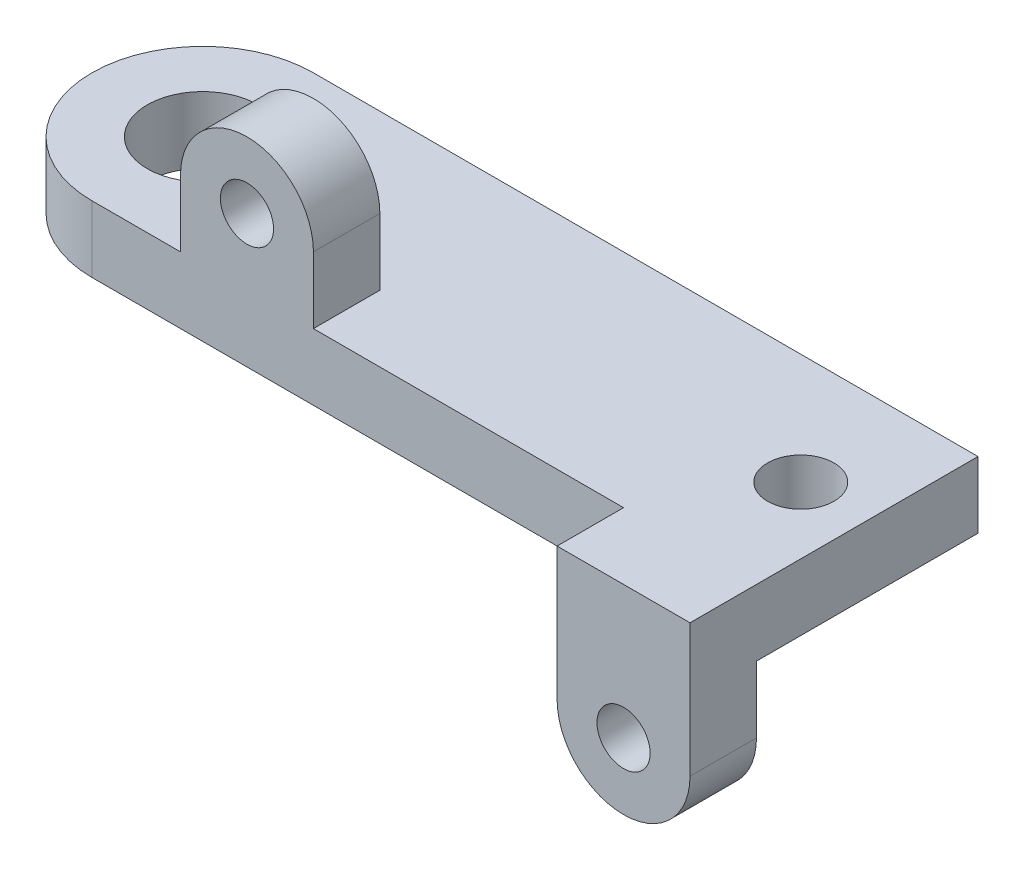
ISO-10303-21;
HEADER;
FILE_DESCRIPTION(('STEP AP214'),'2;1');
FILE_NAME('part.step','',(''),(''),'','','');
FILE_SCHEMA(('AUTOMOTIVE_DESIGN { 1 0 10303 214 1 1 1 1 }'));
ENDSEC;
DATA;
#1=APPLICATION_CONTEXT('core data for automotive mechanical design processes');
#2=APPLICATION_PROTOCOL_DEFINITION('international standard','automotive_design',2000,#1);
#3=PRODUCT_CONTEXT('',#1,'mechanical');
#4=PRODUCT('Part','Part','',(#3));
#5=PRODUCT_RELATED_PRODUCT_CATEGORY('part','',(#4));
#6=PRODUCT_DEFINITION_FORMATION('','',#4);
#7=PRODUCT_DEFINITION_CONTEXT('part definition',#1,'design');
#8=PRODUCT_DEFINITION('design','',#6,#7);
#9=PRODUCT_DEFINITION_SHAPE('','',#8);
#10=(LENGTH_UNIT() NAMED_UNIT(*) SI_UNIT(.MILLI.,.METRE.));
#11=(NAMED_UNIT(*) PLANE_ANGLE_UNIT() SI_UNIT($,.RADIAN.));
#12=(NAMED_UNIT(*) SI_UNIT($,.STERADIAN.) SOLID_ANGLE_UNIT());
#13=UNCERTAINTY_MEASURE_WITH_UNIT(LENGTH_MEASURE(1.E-05),#10,'distance_accuracy_value','');
#14=(GEOMETRIC_REPRESENTATION_CONTEXT(3) GLOBAL_UNCERTAINTY_ASSIGNED_CONTEXT((#13)) GLOBAL_UNIT_ASSIGNED_CONTEXT((#10,
#11,#12)) REPRESENTATION_CONTEXT('',''));
#15=CARTESIAN_POINT('',(0.,0.,0.));
#16=DIRECTION('',(0.,0.,1.));
#17=DIRECTION('',(1.,0.,0.));
#18=AXIS2_PLACEMENT_3D('',#15,#16,#17);
#19=CARTESIAN_POINT('',(120.,-45.,0.));
#20=DIRECTION('',(1.,0.,0.));
#21=DIRECTION('',(0.,0.,-1.));
#22=AXIS2_PLACEMENT_3D('',#19,#20,#21);
#23=PLANE('',#22);
#24=DIRECTION('',(0.,0.,1.));
#25=VECTOR('',#24,1.);
#26=CARTESIAN_POINT('',(120.,-30.,-4.99999999999994));
#27=LINE('',#26,#25);
#28=CARTESIAN_POINT('',(120.,-30.,25.));
#29=VERTEX_POINT('',#28);
#30=CARTESIAN_POINT('',(120.,-30.,40.));
#31=VERTEX_POINT('',#30);
#32=EDGE_CURVE('E165',#29,#31,#27,.T.);
#33=ORIENTED_EDGE('',*,*,#32,.T.);
#34=DIRECTION('',(0.,1.,0.));
#35=VECTOR('',#34,1.);
#36=CARTESIAN_POINT('',(120.,-45.,40.));
#37=LINE('',#36,#35);
#38=CARTESIAN_POINT('',(120.,0.,40.));
#39=VERTEX_POINT('',#38);
#40=EDGE_CURVE('E186',#31,#39,#37,.T.);
#41=ORIENTED_EDGE('',*,*,#40,.T.);
#42=DIRECTION('',(0.,0.,-1.));
#43=VECTOR('',#42,1.);
#44=CARTESIAN_POINT('',(120.,0.,0.));
#45=LINE('',#44,#43);
#46=CARTESIAN_POINT('',(120.,0.,25.));
#47=VERTEX_POINT('',#46);
#48=EDGE_CURVE('E177',#39,#47,#45,.T.);
#49=ORIENTED_EDGE('',*,*,#48,.T.);
#50=DIRECTION('',(0.,1.,0.));
#51=VECTOR('',#50,1.);
#52=CARTESIAN_POINT('',(120.,-45.,25.));
#53=LINE('',#52,#51);
#54=CARTESIAN_POINT('',(120.,-15.,25.));
#55=VERTEX_POINT('',#54);
#56=EDGE_CURVE('E185',#55,#47,#53,.T.);
#57=ORIENTED_EDGE('',*,*,#56,.F.);
#58=EDGE_CURVE('E189',#29,#55,#53,.T.);
#59=ORIENTED_EDGE('',*,*,#58,.F.);
#60=EDGE_LOOP('',(#33,#41,#49,#57,#59));
#61=FACE_BOUND('',#60,.T.);
#62=ADVANCED_FACE('F41',(#61),#23,.F.);
#63=CARTESIAN_POINT('',(0.,-15.,25.));
#64=DIRECTION('',(0.,0.,-1.));
#65=DIRECTION('',(-1.,0.,0.));
#66=AXIS2_PLACEMENT_3D('',#63,#64,#65);
#67=PLANE('',#66);
#68=DIRECTION('',(-1.,0.,0.));
#69=VECTOR('',#68,1.);
#70=CARTESIAN_POINT('',(0.,0.,25.));
#71=LINE('',#70,#69);
#72=CARTESIAN_POINT('',(50.,0.,25.));
#73=VERTEX_POINT('',#72);
#74=EDGE_CURVE('E223',#47,#73,#71,.T.);
#75=ORIENTED_EDGE('',*,*,#74,.T.);
#76=DIRECTION('',(0.,1.,0.));
#77=VECTOR('',#76,1.);
#78=CARTESIAN_POINT('',(50.,-3.36192289386007,25.));
#79=LINE('',#78,#77);
#80=CARTESIAN_POINT('',(50.,15.,25.));
#81=VERTEX_POINT('',#80);
#82=EDGE_CURVE('E147',#73,#81,#79,.T.);
#83=ORIENTED_EDGE('',*,*,#82,.T.);
#84=CARTESIAN_POINT('',(35.,15.,25.));
#85=DIRECTION('',(0.,0.,1.));
#86=DIRECTION('',(1.,0.,0.));
#87=AXIS2_PLACEMENT_3D('',#84,#85,#86);
#88=CIRCLE('',#87,15.);
#89=CARTESIAN_POINT('',(20.,15.,25.));
#90=VERTEX_POINT('',#89);
#91=EDGE_CURVE('E158',#81,#90,#88,.T.);
#92=ORIENTED_EDGE('',*,*,#91,.T.);
#93=DIRECTION('',(0.,-1.,0.));
#94=VECTOR('',#93,1.);
#95=CARTESIAN_POINT('',(20.,15.,25.));
#96=LINE('',#95,#94);
#97=CARTESIAN_POINT('',(20.,0.,25.));
#98=VERTEX_POINT('',#97);
#99=EDGE_CURVE('E57',#90,#98,#96,.T.);
#100=ORIENTED_EDGE('',*,*,#99,.T.);
#101=CARTESIAN_POINT('',(0.,0.,25.));
#102=VERTEX_POINT('',#101);
#103=EDGE_CURVE('E221',#98,#102,#71,.T.);
#104=ORIENTED_EDGE('',*,*,#103,.T.);
#105=DIRECTION('',(0.,1.,0.));
#106=VECTOR('',#105,1.);
#107=CARTESIAN_POINT('',(0.,-15.,25.));
#108=LINE('',#107,#106);
#109=CARTESIAN_POINT('',(0.,-15.,25.));
#110=VERTEX_POINT('',#109);
#111=EDGE_CURVE('E233',#110,#102,#108,.T.);
#112=ORIENTED_EDGE('',*,*,#111,.F.);
#113=DIRECTION('',(-1.,0.,0.));
#114=VECTOR('',#113,1.);
#115=CARTESIAN_POINT('',(0.,-15.,25.));
#116=LINE('',#115,#114);
#117=EDGE_CURVE('E202',#55,#110,#116,.T.);
#118=ORIENTED_EDGE('',*,*,#117,.F.);
#119=ORIENTED_EDGE('',*,*,#56,.T.);
#120=EDGE_LOOP('',(#75,#83,#92,#100,#104,#112,#118,#119));
#121=FACE_BOUND('',#120,.T.);
#122=CARTESIAN_POINT('',(35.,15.,25.));
#123=DIRECTION('',(0.,0.,1.));
#124=DIRECTION('',(1.,0.,0.));
#125=AXIS2_PLACEMENT_3D('',#122,#123,#124);
#126=CIRCLE('',#125,6.);
#127=CARTESIAN_POINT('',(41.,15.,25.));
#128=VERTEX_POINT('',#127);
#129=EDGE_CURVE('E152',#128,#128,#126,.T.);
#130=ORIENTED_EDGE('',*,*,#129,.F.);
#131=EDGE_LOOP('',(#130));
#132=FACE_BOUND('',#131,.T.);
#133=ADVANCED_FACE('F244',(#121,#132),#67,.F.);
#134=CARTESIAN_POINT('',(0.,-15.,-25.));
#135=DIRECTION('',(0.,0.,1.));
#136=DIRECTION('',(1.,0.,0.));
#137=AXIS2_PLACEMENT_3D('',#134,#135,#136);
#138=PLANE('',#137);
#139=DIRECTION('',(1.,0.,0.));
#140=VECTOR('',#139,1.);
#141=CARTESIAN_POINT('',(0.,0.,-25.));
#142=LINE('',#141,#140);
#143=CARTESIAN_POINT('',(0.,0.,-25.));
#144=VERTEX_POINT('',#143);
#145=CARTESIAN_POINT('',(150.,0.,-25.));
#146=VERTEX_POINT('',#145);
#147=EDGE_CURVE('E217',#144,#146,#142,.T.);
#148=ORIENTED_EDGE('',*,*,#147,.T.);
#149=DIRECTION('',(0.,1.,0.));
#150=VECTOR('',#149,1.);
#151=CARTESIAN_POINT('',(150.,-15.,-25.));
#152=LINE('',#151,#150);
#153=CARTESIAN_POINT('',(150.,-15.,-25.));
#154=VERTEX_POINT('',#153);
#155=EDGE_CURVE('E229',#154,#146,#152,.T.);
#156=ORIENTED_EDGE('',*,*,#155,.F.);
#157=DIRECTION('',(1.,0.,0.));
#158=VECTOR('',#157,1.);
#159=CARTESIAN_POINT('',(0.,-15.,-25.));
#160=LINE('',#159,#158);
#161=CARTESIAN_POINT('',(0.,-15.,-25.));
#162=VERTEX_POINT('',#161);
#163=EDGE_CURVE('E200',#162,#154,#160,.T.);
#164=ORIENTED_EDGE('',*,*,#163,.F.);
#165=DIRECTION('',(0.,1.,0.));
#166=VECTOR('',#165,1.);
#167=CARTESIAN_POINT('',(0.,-15.,-25.));
#168=LINE('',#167,#166);
#169=EDGE_CURVE('E215',#162,#144,#168,.T.);
#170=ORIENTED_EDGE('',*,*,#169,.T.);
#171=EDGE_LOOP('',(#148,#156,#164,#170));
#172=FACE_BOUND('',#171,.T.);
#173=ADVANCED_FACE('F285',(#172),#138,.F.);
#174=CARTESIAN_POINT('',(150.,-15.,0.));
#175=DIRECTION('',(-1.,0.,0.));
#176=DIRECTION('',(0.,0.,1.));
#177=AXIS2_PLACEMENT_3D('',#174,#175,#176);
#178=PLANE('',#177);
#179=DIRECTION('',(0.,1.,0.));
#180=VECTOR('',#179,1.);
#181=CARTESIAN_POINT('',(150.,-45.,40.));
#182=LINE('',#181,#180);
#183=CARTESIAN_POINT('',(150.,-30.,40.0000000000001));
#184=VERTEX_POINT('',#183);
#185=CARTESIAN_POINT('',(150.,0.,40.));
#186=VERTEX_POINT('',#185);
#187=EDGE_CURVE('E188',#184,#186,#182,.T.);
#188=ORIENTED_EDGE('',*,*,#187,.F.);
#189=DIRECTION('',(0.,0.,1.));
#190=VECTOR('',#189,1.);
#191=CARTESIAN_POINT('',(150.,-30.,-4.99999999999994));
#192=LINE('',#191,#190);
#193=CARTESIAN_POINT('',(150.,-30.,25.));
#194=VERTEX_POINT('',#193);
#195=EDGE_CURVE('E163',#194,#184,#192,.T.);
#196=ORIENTED_EDGE('',*,*,#195,.F.);
#197=DIRECTION('',(0.,1.,0.));
#198=VECTOR('',#197,1.);
#199=CARTESIAN_POINT('',(150.,-45.,25.));
#200=LINE('',#199,#198);
#201=CARTESIAN_POINT('',(150.,-15.,25.));
#202=VERTEX_POINT('',#201);
#203=EDGE_CURVE('E181',#194,#202,#200,.T.);
#204=ORIENTED_EDGE('',*,*,#203,.T.);
#205=DIRECTION('',(0.,0.,1.));
#206=VECTOR('',#205,1.);
#207=CARTESIAN_POINT('',(150.,-15.,0.));
#208=LINE('',#207,#206);
#209=EDGE_CURVE('E207',#154,#202,#208,.T.);
#210=ORIENTED_EDGE('',*,*,#209,.F.);
#211=ORIENTED_EDGE('',*,*,#155,.T.);
#212=DIRECTION('',(0.,0.,1.));
#213=VECTOR('',#212,1.);
#214=CARTESIAN_POINT('',(150.,0.,0.));
#215=LINE('',#214,#213);
#216=EDGE_CURVE('E198',#146,#186,#215,.T.);
#217=ORIENTED_EDGE('',*,*,#216,.T.);
#218=EDGE_LOOP('',(#188,#196,#204,#210,#211,#217));
#219=FACE_BOUND('',#218,.T.);
#220=ADVANCED_FACE('F298',(#219),#178,.F.);
#221=CARTESIAN_POINT('',(0.,-15.,0.));
#222=DIRECTION('',(0.,1.,0.));
#223=DIRECTION('',(0.,0.,1.));
#224=AXIS2_PLACEMENT_3D('',#221,#222,#223);
#225=CYLINDRICAL_SURFACE('',#224,12.5);
#226=CARTESIAN_POINT('',(0.,-15.,0.));
#227=DIRECTION('',(0.,1.,0.));
#228=DIRECTION('',(0.,0.,1.));
#229=AXIS2_PLACEMENT_3D('',#226,#227,#228);
#230=CIRCLE('',#229,12.5);
#231=CARTESIAN_POINT('',(0.,-15.,12.5));
#232=VERTEX_POINT('',#231);
#233=EDGE_CURVE('E191',#232,#232,#230,.T.);
#234=ORIENTED_EDGE('',*,*,#233,.F.);
#235=EDGE_LOOP('',(#234));
#236=FACE_BOUND('',#235,.T.);
#237=CARTESIAN_POINT('',(0.,0.,0.));
#238=DIRECTION('',(0.,1.,0.));
#239=DIRECTION('',(0.,0.,1.));
#240=AXIS2_PLACEMENT_3D('',#237,#238,#239);
#241=CIRCLE('',#240,12.5);
#242=CARTESIAN_POINT('',(0.,0.,12.5));
#243=VERTEX_POINT('',#242);
#244=EDGE_CURVE('E214',#243,#243,#241,.T.);
#245=ORIENTED_EDGE('',*,*,#244,.T.);
#246=EDGE_LOOP('',(#245));
#247=FACE_BOUND('',#246,.T.);
#248=ADVANCED_FACE('F300',(#236,#247),#225,.F.);
#249=CARTESIAN_POINT('',(135.,-15.,0.));
#250=DIRECTION('',(0.,1.,0.));
#251=DIRECTION('',(0.,0.,1.));
#252=AXIS2_PLACEMENT_3D('',#249,#250,#251);
#253=CYLINDRICAL_SURFACE('',#252,7.50000000000001);
#254=CARTESIAN_POINT('',(135.,-15.,0.));
#255=DIRECTION('',(0.,1.,0.));
#256=DIRECTION('',(0.,0.,1.));
#257=AXIS2_PLACEMENT_3D('',#254,#255,#256);
#258=CIRCLE('',#257,7.50000000000001);
#259=CARTESIAN_POINT('',(135.,-15.,7.50000000000002));
#260=VERTEX_POINT('',#259);
#261=EDGE_CURVE('E195',#260,#260,#258,.T.);
#262=ORIENTED_EDGE('',*,*,#261,.F.);
#263=EDGE_LOOP('',(#262));
#264=FACE_BOUND('',#263,.T.);
#265=CARTESIAN_POINT('',(135.,0.,0.));
#266=DIRECTION('',(0.,1.,0.));
#267=DIRECTION('',(0.,0.,1.));
#268=AXIS2_PLACEMENT_3D('',#265,#266,#267);
#269=CIRCLE('',#268,7.50000000000001);
#270=CARTESIAN_POINT('',(135.,0.,7.50000000000002));
#271=VERTEX_POINT('',#270);
#272=EDGE_CURVE('E183',#271,#271,#269,.T.);
#273=ORIENTED_EDGE('',*,*,#272,.T.);
#274=EDGE_LOOP('',(#273));
#275=FACE_BOUND('',#274,.T.);
#276=ADVANCED_FACE('F43',(#264,#275),#253,.F.);
#277=CARTESIAN_POINT('',(0.,-15.,0.));
#278=DIRECTION('',(0.,1.,0.));
#279=DIRECTION('',(0.,0.,1.));
#280=AXIS2_PLACEMENT_3D('',#277,#278,#279);
#281=CYLINDRICAL_SURFACE('',#280,25.);
#282=CARTESIAN_POINT('',(0.,0.,0.));
#283=DIRECTION('',(0.,1.,0.));
#284=DIRECTION('',(0.,0.,1.));
#285=AXIS2_PLACEMENT_3D('',#282,#283,#284);
#286=CIRCLE('',#285,25.);
#287=EDGE_CURVE('E222',#144,#102,#286,.T.);
#288=ORIENTED_EDGE('',*,*,#287,.F.);
#289=ORIENTED_EDGE('',*,*,#169,.F.);
#290=CARTESIAN_POINT('',(0.,-15.,0.));
#291=DIRECTION('',(0.,1.,0.));
#292=DIRECTION('',(0.,0.,1.));
#293=AXIS2_PLACEMENT_3D('',#290,#291,#292);
#294=CIRCLE('',#293,25.);
#295=EDGE_CURVE('E205',#162,#110,#294,.T.);
#296=ORIENTED_EDGE('',*,*,#295,.T.);
#297=ORIENTED_EDGE('',*,*,#111,.T.);
#298=EDGE_LOOP('',(#288,#289,#296,#297));
#299=FACE_BOUND('',#298,.T.);
#300=ADVANCED_FACE('F249',(#299),#281,.T.);
#301=CARTESIAN_POINT('',(0.,-15.,0.));
#302=DIRECTION('',(0.,1.,0.));
#303=DIRECTION('',(0.,0.,1.));
#304=AXIS2_PLACEMENT_3D('',#301,#302,#303);
#305=PLANE('',#304);
#306=ORIENTED_EDGE('',*,*,#261,.T.);
#307=EDGE_LOOP('',(#306));
#308=FACE_BOUND('',#307,.T.);
#309=ORIENTED_EDGE('',*,*,#233,.T.);
#310=EDGE_LOOP('',(#309));
#311=FACE_BOUND('',#310,.T.);
#312=ORIENTED_EDGE('',*,*,#163,.T.);
#313=ORIENTED_EDGE('',*,*,#209,.T.);
#314=EDGE_CURVE('E206',#202,#55,#116,.T.);
#315=ORIENTED_EDGE('',*,*,#314,.T.);
#316=ORIENTED_EDGE('',*,*,#117,.T.);
#317=ORIENTED_EDGE('',*,*,#295,.F.);
#318=EDGE_LOOP('',(#312,#313,#315,#316,#317));
#319=FACE_BOUND('',#318,.T.);
#320=ADVANCED_FACE('F251',(#308,#311,#319),#305,.F.);
#321=CARTESIAN_POINT('',(0.,0.,0.));
#322=DIRECTION('',(0.,1.,0.));
#323=DIRECTION('',(0.,0.,1.));
#324=AXIS2_PLACEMENT_3D('',#321,#322,#323);
#325=PLANE('',#324);
#326=DIRECTION('',(0.,0.,-1.));
#327=VECTOR('',#326,1.);
#328=CARTESIAN_POINT('',(50.,0.,0.));
#329=LINE('',#328,#327);
#330=CARTESIAN_POINT('',(50.,0.,10.));
#331=VERTEX_POINT('',#330);
#332=EDGE_CURVE('E11',#73,#331,#329,.T.);
#333=ORIENTED_EDGE('',*,*,#332,.F.);
#334=ORIENTED_EDGE('',*,*,#74,.F.);
#335=ORIENTED_EDGE('',*,*,#48,.F.);
#336=DIRECTION('',(-1.,0.,0.));
#337=VECTOR('',#336,1.);
#338=CARTESIAN_POINT('',(0.,0.,40.0000000000001));
#339=LINE('',#338,#337);
#340=EDGE_CURVE('E179',#186,#39,#339,.T.);
#341=ORIENTED_EDGE('',*,*,#340,.F.);
#342=ORIENTED_EDGE('',*,*,#216,.F.);
#343=ORIENTED_EDGE('',*,*,#147,.F.);
#344=ORIENTED_EDGE('',*,*,#287,.T.);
#345=ORIENTED_EDGE('',*,*,#103,.F.);
#346=DIRECTION('',(0.,0.,1.));
#347=VECTOR('',#346,1.);
#348=CARTESIAN_POINT('',(20.,0.,0.));
#349=LINE('',#348,#347);
#350=CARTESIAN_POINT('',(20.,0.,10.));
#351=VERTEX_POINT('',#350);
#352=EDGE_CURVE('E47',#351,#98,#349,.T.);
#353=ORIENTED_EDGE('',*,*,#352,.F.);
#354=DIRECTION('',(1.,0.,0.));
#355=VECTOR('',#354,1.);
#356=CARTESIAN_POINT('',(0.,0.,10.));
#357=LINE('',#356,#355);
#358=EDGE_CURVE('E144',#351,#331,#357,.T.);
#359=ORIENTED_EDGE('',*,*,#358,.T.);
#360=EDGE_LOOP('',(#333,#334,#335,#341,#342,#343,#344,#345,#353,#359));
#361=FACE_BOUND('',#360,.T.);
#362=ORIENTED_EDGE('',*,*,#272,.F.);
#363=EDGE_LOOP('',(#362));
#364=FACE_BOUND('',#363,.T.);
#365=ORIENTED_EDGE('',*,*,#244,.F.);
#366=EDGE_LOOP('',(#365));
#367=FACE_BOUND('',#366,.T.);
#368=ADVANCED_FACE('F238',(#361,#364,#367),#325,.T.);
#369=CARTESIAN_POINT('',(0.,-45.,25.));
#370=DIRECTION('',(0.,0.,1.));
#371=DIRECTION('',(1.,0.,0.));
#372=AXIS2_PLACEMENT_3D('',#369,#370,#371);
#373=PLANE('',#372);
#374=CARTESIAN_POINT('',(135.,-30.,25.));
#375=DIRECTION('',(0.,0.,1.));
#376=DIRECTION('',(1.,0.,0.));
#377=AXIS2_PLACEMENT_3D('',#374,#375,#376);
#378=CIRCLE('',#377,6.00000000000002);
#379=CARTESIAN_POINT('',(141.,-30.,25.));
#380=VERTEX_POINT('',#379);
#381=EDGE_CURVE('E171',#380,#380,#378,.T.);
#382=ORIENTED_EDGE('',*,*,#381,.T.);
#383=EDGE_LOOP('',(#382));
#384=FACE_BOUND('',#383,.T.);
#385=ORIENTED_EDGE('',*,*,#203,.F.);
#386=CARTESIAN_POINT('',(135.,-30.,25.));
#387=DIRECTION('',(0.,0.,1.));
#388=DIRECTION('',(1.,0.,0.));
#389=AXIS2_PLACEMENT_3D('',#386,#387,#388);
#390=CIRCLE('',#389,15.);
#391=EDGE_CURVE('E173',#194,#29,#390,.F.);
#392=ORIENTED_EDGE('',*,*,#391,.T.);
#393=ORIENTED_EDGE('',*,*,#58,.T.);
#394=ORIENTED_EDGE('',*,*,#314,.F.);
#395=EDGE_LOOP('',(#385,#392,#393,#394));
#396=FACE_BOUND('',#395,.T.);
#397=ADVANCED_FACE('F288',(#384,#396),#373,.F.);
#398=CARTESIAN_POINT('',(0.,-45.,40.0000000000001));
#399=DIRECTION('',(0.,0.,-1.));
#400=DIRECTION('',(-1.,0.,0.));
#401=AXIS2_PLACEMENT_3D('',#398,#399,#400);
#402=PLANE('',#401);
#403=CARTESIAN_POINT('',(135.,-30.,40.0000000000001));
#404=DIRECTION('',(0.,0.,1.));
#405=DIRECTION('',(1.,0.,0.));
#406=AXIS2_PLACEMENT_3D('',#403,#404,#405);
#407=CIRCLE('',#406,6.00000000000002);
#408=CARTESIAN_POINT('',(141.,-30.,40.0000000000001));
#409=VERTEX_POINT('',#408);
#410=EDGE_CURVE('E169',#409,#409,#407,.T.);
#411=ORIENTED_EDGE('',*,*,#410,.F.);
#412=EDGE_LOOP('',(#411));
#413=FACE_BOUND('',#412,.T.);
#414=ORIENTED_EDGE('',*,*,#40,.F.);
#415=CARTESIAN_POINT('',(135.,-30.,40.0000000000001));
#416=DIRECTION('',(0.,0.,-1.));
#417=DIRECTION('',(1.,0.,0.));
#418=AXIS2_PLACEMENT_3D('',#415,#416,#417);
#419=CIRCLE('',#418,15.);
#420=EDGE_CURVE('E62',#184,#31,#419,.T.);
#421=ORIENTED_EDGE('',*,*,#420,.F.);
#422=ORIENTED_EDGE('',*,*,#187,.T.);
#423=ORIENTED_EDGE('',*,*,#340,.T.);
#424=EDGE_LOOP('',(#414,#421,#422,#423));
#425=FACE_BOUND('',#424,.T.);
#426=ADVANCED_FACE('F287',(#413,#425),#402,.F.);
#427=CARTESIAN_POINT('',(135.,-30.,-4.99999999999994));
#428=DIRECTION('',(0.,0.,1.));
#429=DIRECTION('',(1.,0.,0.));
#430=AXIS2_PLACEMENT_3D('',#427,#428,#429);
#431=CYLINDRICAL_SURFACE('',#430,15.);
#432=ORIENTED_EDGE('',*,*,#195,.T.);
#433=ORIENTED_EDGE('',*,*,#420,.T.);
#434=ORIENTED_EDGE('',*,*,#32,.F.);
#435=ORIENTED_EDGE('',*,*,#391,.F.);
#436=EDGE_LOOP('',(#432,#433,#434,#435));
#437=FACE_BOUND('',#436,.T.);
#438=ADVANCED_FACE('F380',(#437),#431,.T.);
#439=CARTESIAN_POINT('',(135.,-30.,-4.99999999999994));
#440=DIRECTION('',(0.,0.,1.));
#441=DIRECTION('',(1.,0.,0.));
#442=AXIS2_PLACEMENT_3D('',#439,#440,#441);
#443=CYLINDRICAL_SURFACE('',#442,6.00000000000002);
#444=CARTESIAN_POINT('',(141.,-30.,40.0000000000001));
#445=CARTESIAN_POINT('',(141.,-30.,39.84375));
#446=CARTESIAN_POINT('',(141.,-30.,39.6875000000001));
#447=CARTESIAN_POINT('',(141.,-30.,39.3750000000001));
#448=CARTESIAN_POINT('',(141.,-30.,39.21875));
#449=CARTESIAN_POINT('',(141.,-30.,38.90625));
#450=CARTESIAN_POINT('',(141.,-30.,38.7500000000001));
#451=CARTESIAN_POINT('',(141.,-30.,38.4375));
#452=CARTESIAN_POINT('',(141.,-30.,38.28125));
#453=CARTESIAN_POINT('',(141.,-30.,37.96875));
#454=CARTESIAN_POINT('',(141.,-30.,37.8125));
#455=CARTESIAN_POINT('',(141.,-30.,37.5));
#456=CARTESIAN_POINT('',(141.,-30.,37.34375));
#457=CARTESIAN_POINT('',(141.,-30.,37.03125));
#458=CARTESIAN_POINT('',(141.,-30.,36.875));
#459=CARTESIAN_POINT('',(141.,-30.,36.5625));
#460=CARTESIAN_POINT('',(141.,-30.,36.40625));
#461=CARTESIAN_POINT('',(141.,-30.,36.09375));
#462=CARTESIAN_POINT('',(141.,-30.,35.9375));
#463=CARTESIAN_POINT('',(141.,-30.,35.625));
#464=CARTESIAN_POINT('',(141.,-30.,35.46875));
#465=CARTESIAN_POINT('',(141.,-30.,35.15625));
#466=CARTESIAN_POINT('',(141.,-30.,35.));
#467=CARTESIAN_POINT('',(141.,-30.,34.6875));
#468=CARTESIAN_POINT('',(141.,-30.,34.53125));
#469=CARTESIAN_POINT('',(141.,-30.,34.21875));
#470=CARTESIAN_POINT('',(141.,-30.,34.0625));
#471=CARTESIAN_POINT('',(141.,-30.,33.75));
#472=CARTESIAN_POINT('',(141.,-30.,33.59375));
#473=CARTESIAN_POINT('',(141.,-30.,33.28125));
#474=CARTESIAN_POINT('',(141.,-30.,33.125));
#475=CARTESIAN_POINT('',(141.,-30.,32.8125));
#476=CARTESIAN_POINT('',(141.,-30.,32.65625));
#477=CARTESIAN_POINT('',(141.,-30.,32.34375));
#478=CARTESIAN_POINT('',(141.,-30.,32.1875));
#479=CARTESIAN_POINT('',(141.,-30.,31.875));
#480=CARTESIAN_POINT('',(141.,-30.,31.71875));
#481=CARTESIAN_POINT('',(141.,-30.,31.40625));
#482=CARTESIAN_POINT('',(141.,-30.,31.25));
#483=CARTESIAN_POINT('',(141.,-30.,30.9375));
#484=CARTESIAN_POINT('',(141.,-30.,30.78125));
#485=CARTESIAN_POINT('',(141.,-30.,30.46875));
#486=CARTESIAN_POINT('',(141.,-30.,30.3125));
#487=CARTESIAN_POINT('',(141.,-30.,30.));
#488=CARTESIAN_POINT('',(141.,-30.,29.84375));
#489=CARTESIAN_POINT('',(141.,-30.,29.53125));
#490=CARTESIAN_POINT('',(141.,-30.,29.375));
#491=CARTESIAN_POINT('',(141.,-30.,29.0625));
#492=CARTESIAN_POINT('',(141.,-30.,28.90625));
#493=CARTESIAN_POINT('',(141.,-30.,28.59375));
#494=CARTESIAN_POINT('',(141.,-30.,28.4375));
#495=CARTESIAN_POINT('',(141.,-30.,28.125));
#496=CARTESIAN_POINT('',(141.,-30.,27.96875));
#497=CARTESIAN_POINT('',(141.,-30.,27.65625));
#498=CARTESIAN_POINT('',(141.,-30.,27.5));
#499=CARTESIAN_POINT('',(141.,-30.,27.1875));
#500=CARTESIAN_POINT('',(141.,-30.,27.03125));
#501=CARTESIAN_POINT('',(141.,-30.,26.71875));
#502=CARTESIAN_POINT('',(141.,-30.,26.5625));
#503=CARTESIAN_POINT('',(141.,-30.,26.25));
#504=CARTESIAN_POINT('',(141.,-30.,26.09375));
#505=CARTESIAN_POINT('',(141.,-30.,25.78125));
#506=CARTESIAN_POINT('',(141.,-30.,25.625));
#507=CARTESIAN_POINT('',(141.,-30.,25.3125));
#508=CARTESIAN_POINT('',(141.,-30.,25.15625));
#509=CARTESIAN_POINT('',(141.,-30.,25.));
#510=B_SPLINE_CURVE_WITH_KNOTS('',3,(#444,#445,#446,#447,#448,#449,#450,#451,#452,#453,#454,
#455,#456,#457,#458,#459,#460,#461,#462,#463,#464,#465,#466,#467,#468,#469,#470,#471,#472,#473,
#474,#475,#476,#477,#478,#479,#480,#481,#482,#483,#484,#485,#486,#487,#488,#489,#490,#491,#492,
#493,#494,#495,#496,#497,#498,#499,#500,#501,#502,#503,#504,#505,#506,#507,#508,#509),
.UNSPECIFIED.,.F.,.F.,(4,2,2,2,2,2,2,2,2,2,2,2,2,2,2,2,2,2,2,2,2,2,2,2,2,2,2,2,2,2,2,2,4),(0.,
0.468750000000004,0.937500000000001,1.40625,1.87500000000001,2.34375000000001,2.81250000000001,
3.28125000000001,3.75000000000002,4.21875000000002,4.68750000000002,5.15625000000002,
5.62500000000003,6.09375000000002,6.56250000000003,7.03125000000003,7.50000000000003,
7.96875000000003,8.43750000000004,8.90625000000004,9.37500000000004,9.84375000000004,10.3125,
10.78125,11.25,11.71875,12.1875000000001,12.65625,13.1250000000001,13.5937500000001,
14.0625000000001,14.5312500000001,15.0000000000001),.UNSPECIFIED.);
#511=EDGE_CURVE('BSEAM275',#409,#380,#510,.T.);
#512=ORIENTED_EDGE('',*,*,#410,.T.);
#513=ORIENTED_EDGE('',*,*,#381,.F.);
#514=ORIENTED_EDGE('',*,*,#511,.T.);
#515=ORIENTED_EDGE('',*,*,#511,.F.);
#516=EDGE_LOOP('',(#512,#514,#513,#515));
#517=FACE_BOUND('',#516,.T.);
#518=ADVANCED_FACE('F275',(#517),#443,.F.);
#519=CARTESIAN_POINT('',(35.,15.,10.));
#520=DIRECTION('',(0.,0.,1.));
#521=DIRECTION('',(1.,0.,0.));
#522=AXIS2_PLACEMENT_3D('',#519,#520,#521);
#523=CYLINDRICAL_SURFACE('',#522,15.);
#524=ORIENTED_EDGE('',*,*,#91,.F.);
#525=DIRECTION('',(0.,0.,1.));
#526=VECTOR('',#525,1.);
#527=CARTESIAN_POINT('',(50.,15.,10.));
#528=LINE('',#527,#526);
#529=CARTESIAN_POINT('',(50.,15.,10.));
#530=VERTEX_POINT('',#529);
#531=EDGE_CURVE('E134',#530,#81,#528,.T.);
#532=ORIENTED_EDGE('',*,*,#531,.F.);
#533=CARTESIAN_POINT('',(35.,15.,10.));
#534=DIRECTION('',(0.,0.,1.));
#535=DIRECTION('',(1.,0.,0.));
#536=AXIS2_PLACEMENT_3D('',#533,#534,#535);
#537=CIRCLE('',#536,15.);
#538=CARTESIAN_POINT('',(20.,15.,10.));
#539=VERTEX_POINT('',#538);
#540=EDGE_CURVE('E141',#530,#539,#537,.T.);
#541=ORIENTED_EDGE('',*,*,#540,.T.);
#542=DIRECTION('',(0.,0.,1.));
#543=VECTOR('',#542,1.);
#544=CARTESIAN_POINT('',(20.,15.,10.));
#545=LINE('',#544,#543);
#546=EDGE_CURVE('E130',#539,#90,#545,.T.);
#547=ORIENTED_EDGE('',*,*,#546,.T.);
#548=EDGE_LOOP('',(#524,#532,#541,#547));
#549=FACE_BOUND('',#548,.T.);
#550=ADVANCED_FACE('F146',(#549),#523,.T.);
#551=CARTESIAN_POINT('',(50.,-3.36192289386007,10.));
#552=DIRECTION('',(1.,0.,0.));
#553=DIRECTION('',(0.,0.,-1.));
#554=AXIS2_PLACEMENT_3D('',#551,#552,#553);
#555=PLANE('',#554);
#556=ORIENTED_EDGE('',*,*,#82,.F.);
#557=ORIENTED_EDGE('',*,*,#332,.T.);
#558=DIRECTION('',(0.,1.,0.));
#559=VECTOR('',#558,1.);
#560=CARTESIAN_POINT('',(50.,-3.36192289386007,10.));
#561=LINE('',#560,#559);
#562=EDGE_CURVE('E137',#331,#530,#561,.T.);
#563=ORIENTED_EDGE('',*,*,#562,.T.);
#564=ORIENTED_EDGE('',*,*,#531,.T.);
#565=EDGE_LOOP('',(#556,#557,#563,#564));
#566=FACE_BOUND('',#565,.T.);
#567=ADVANCED_FACE('F262',(#566),#555,.T.);
#568=CARTESIAN_POINT('',(20.,15.,10.));
#569=DIRECTION('',(-1.,0.,0.));
#570=DIRECTION('',(0.,0.,1.));
#571=AXIS2_PLACEMENT_3D('',#568,#569,#570);
#572=PLANE('',#571);
#573=DIRECTION('',(0.,-1.,0.));
#574=VECTOR('',#573,1.);
#575=CARTESIAN_POINT('',(20.,15.,10.));
#576=LINE('',#575,#574);
#577=EDGE_CURVE('E128',#539,#351,#576,.T.);
#578=ORIENTED_EDGE('',*,*,#577,.T.);
#579=ORIENTED_EDGE('',*,*,#352,.T.);
#580=ORIENTED_EDGE('',*,*,#99,.F.);
#581=ORIENTED_EDGE('',*,*,#546,.F.);
#582=EDGE_LOOP('',(#578,#579,#580,#581));
#583=FACE_BOUND('',#582,.T.);
#584=ADVANCED_FACE('F129',(#583),#572,.T.);
#585=CARTESIAN_POINT('',(35.,15.,10.));
#586=DIRECTION('',(0.,0.,1.));
#587=DIRECTION('',(1.,0.,0.));
#588=AXIS2_PLACEMENT_3D('',#585,#586,#587);
#589=PLANE('',#588);
#590=ORIENTED_EDGE('',*,*,#358,.F.);
#591=ORIENTED_EDGE('',*,*,#577,.F.);
#592=ORIENTED_EDGE('',*,*,#540,.F.);
#593=ORIENTED_EDGE('',*,*,#562,.F.);
#594=EDGE_LOOP('',(#590,#591,#592,#593));
#595=FACE_BOUND('',#594,.T.);
#596=CARTESIAN_POINT('',(35.,15.,10.));
#597=DIRECTION('',(0.,0.,1.));
#598=DIRECTION('',(1.,0.,0.));
#599=AXIS2_PLACEMENT_3D('',#596,#597,#598);
#600=CIRCLE('',#599,6.);
#601=CARTESIAN_POINT('',(41.,15.,10.));
#602=VERTEX_POINT('',#601);
#603=EDGE_CURVE('E159',#602,#602,#600,.T.);
#604=ORIENTED_EDGE('',*,*,#603,.T.);
#605=EDGE_LOOP('',(#604));
#606=FACE_BOUND('',#605,.T.);
#607=ADVANCED_FACE('F136',(#595,#606),#589,.F.);
#608=CARTESIAN_POINT('',(35.,15.,10.));
#609=DIRECTION('',(0.,0.,1.));
#610=DIRECTION('',(1.,0.,0.));
#611=AXIS2_PLACEMENT_3D('',#608,#609,#610);
#612=CYLINDRICAL_SURFACE('',#611,6.);
#613=ORIENTED_EDGE('',*,*,#603,.F.);
#614=EDGE_LOOP('',(#613));
#615=FACE_BOUND('',#614,.T.);
#616=ORIENTED_EDGE('',*,*,#129,.T.);
#617=EDGE_LOOP('',(#616));
#618=FACE_BOUND('',#617,.T.);
#619=ADVANCED_FACE('F425',(#615,#618),#612,.F.);
#620=CLOSED_SHELL('',(#62,#133,#173,#220,#248,#276,#300,#320,#368,#397,#426,#438,#518,#550,#567,
#584,#607,#619));
#621=MANIFOLD_SOLID_BREP('B2',#620);
#622=ADVANCED_BREP_SHAPE_REPRESENTATION('',(#18,#621),#14);
#623=SHAPE_DEFINITION_REPRESENTATION(#9,#622);
ENDSEC;
END-ISO-10303-21;
